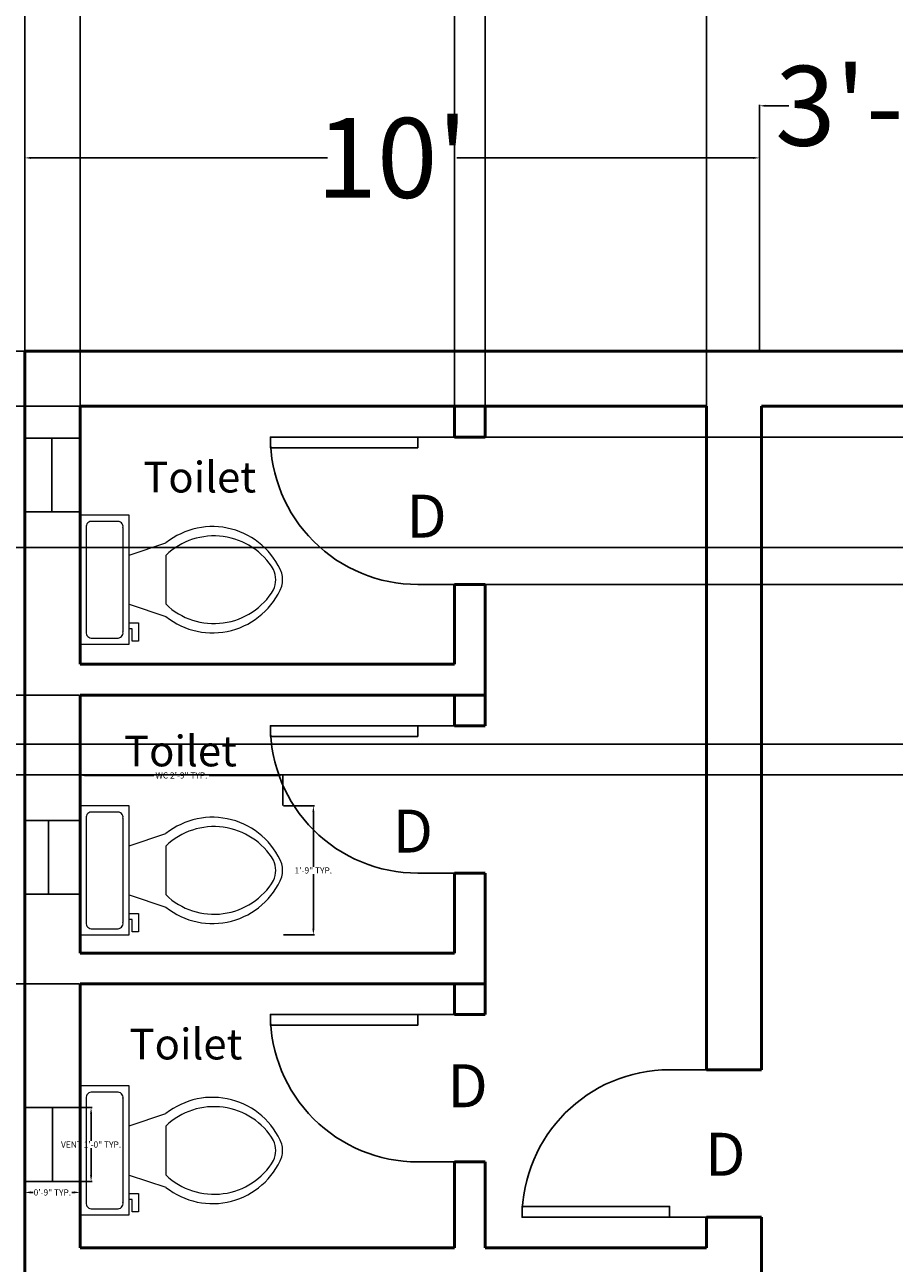
# Model space of a CAD drawing. Units: inches. Extents: x -364 to 705, y -52 to 1250.
# Tile 25 of 34: x 29 to 170, y 838 to 1039. Entities that reach past the tile are written whole.
import ezdxf

# ---------------------------------------------------------------- set-up
doc = ezdxf.new("R2010")
doc.units = ezdxf.units.IN
doc.header["$MEASUREMENT"] = 0
for name, color, linetype, lineweight in [('A-ANNO-DIMS', 4, 'Continuous', 18), ('A-ANNO-IDEN', 1, 'Continuous', 18), ('A-AREA-IDEN', 3, 'Continuous', 18), ('A-DOOR', 1, 'Continuous', 25), ('A-FLOR-FIXT', 9, 'Continuous', 18), ('A-GLAZ', 4, 'Continuous', 25), ('A-WALL', 41, 'Continuous', 50)]:
    doc.layers.add(name, color=color, linetype=linetype, lineweight=lineweight)
doc.styles.get("Standard").update_dxf_attribs({"font": 'arial.ttf'})
doc.dimstyles.get("Standard").update_dxf_attribs({"dimtxt": 1, "dimasz": 1, "dimexe": 0.18, "dimexo": 0.0625, "dimgap": 0.09, "dimtad": 0, "dimtih": 1, "dimtoh": 1, "dimdec": 0, "dimzin": 0, "dimdsep": 46, "dimlunit": 3, "dimtxsty": 'Standard', "dimcen": 0.09, "dimadec": 0, "dimazin": 0, "dimtfac": 1, "dimtdec": 0, "dimtofl": 0, "dimtmove": 0, "dimatfit": 3, "dimfxl": 1, "dimtolj": 1, "dimtzin": 0, "dimarcsym": 0})

# ---------------------------------------------------------------- blocks, each defined once
blk = doc.blocks.new('*U15')
for p, q in [((0, 0), (0, 6)), ((24, 0), (24, 6))]:
    blk.add_line(p, q)
blk.add_lwpolyline([(0, 0), (0, -24), (1.75, -24), (1.75, 0)], close=True)
blk.add_arc((0, 0), 24, 270, 0)
blk = doc.blocks.new('*U16')
for p, q in [((-24, 0), (-24, 6)), ((0, 0), (0, 6))]:
    blk.add_line(p, q)
blk.add_lwpolyline([(0, 0), (0, -24), (-1.75, -24), (-1.75, 0)], close=True)
blk.add_arc((0, 0), 24, 180, 270)
blk = doc.blocks.new('Toilet - top')
for p, q in [((9.5, -6), (9.5, -2)), ((-8, -8.5), (-8, -8)), ((-7, -8), (-7, -9.5)), ((-4, -8), (-6, -14)), ((4, -8), (6, -14)), ((-10, -8.5), (-8, -8.5)), ((-10, -9.5), (-10, -8.5)), ((-7, -9.5), (-10, -9.5)), ((4, -14), (-4, -14))]:
    blk.add_line(p, q)
blk.add_lwpolyline([(10.5, -8), (10.5, 0), (-10.5, 0), (-10.5, -8)], close=True)
for points in [[(-9.5, -2), (-9.5, -6)], [(8.5, -1), (-8.5, -1)], [(-8.5, -7), (8.5, -7)]]:
    blk.add_lwpolyline(points)
for centre, radius, start, end in [((-8.62, -1.88), 0.884, 81.8699, 188.1301), ((8.62, -1.88), 0.884, 351.8699, 98.1301), ((-8.62, -6.12), 0.884, 171.8699, 278.1301), ((8.62, -6.12), 0.884, 261.8699, 8.1301), ((3.52, -21.58), 12.17, 141.4691, 247.9714), ((4.2, -21.82), 11.33, 136.3677, 238.9468), ((-3.52, -21.58), 12.17, 292.0284, 38.5307), ((-4.2, -21.82), 11.33, 301.053, 43.6321), ((0, -27.88), 4, 245.7318, 294.2682), ((0, -29), 4, 254.8605, 285.1395)]:
    blk.add_arc(centre, radius, start, end)
blk = doc.blocks.new('*D19')
at = {"layer": 'A-ANNO-DIMS', "color": 0, "lineweight": -2, "transparency": 16777216}
for p, q in [((28.52, 986.11), (-248.33, 986.11)), ((-248.15, 985.11), (-248.15, 574.22)), ((-248.15, 149.87), (-248.15, 560.77)), ((28.52, 148.87), (-248.33, 148.87))]:
    blk.add_line(p, q, dxfattribs=at)
at = {"layer": 'A-ANNO-DIMS', "color": 0, "transparency": 16777216}
for points in [[(-248.32, 985.11), (-247.99, 985.11), (-248.15, 986.11)], [(-248.32, 149.87), (-247.99, 149.87), (-248.15, 148.87)]]:
    blk.add_solid(points, dxfattribs=at)
at = {"layer": 'Defpoints', "color": 0, "transparency": 16777216}
for p in [(28.58, 986.11), (-248.15, 148.87), (28.58, 148.87)]:
    blk.add_point(p, dxfattribs=at)
at = {"layer": 'A-ANNO-DIMS', "color": 0, "transparency": 16777216, "insert": (-248.15, 567.49), "char_height": 1, "attachment_point": 5}
blk.add_mtext('\\A1;{\\H13x;69\'-9"}', dxfattribs=at)
blk = doc.blocks.new('*D20')
at = {"layer": 'A-ANNO-DIMS', "color": 0, "lineweight": -2, "transparency": 16777216}
for p, q in [((28.52, 986.11), (-188.21, 986.11)), ((-188.03, 985.11), (-188.03, 917.23)), ((-188.03, 836.11), (-188.03, 904)), ((37.52, 835.11), (-188.21, 835.11))]:
    blk.add_line(p, q, dxfattribs=at)
at = {"layer": 'A-ANNO-DIMS', "color": 0, "transparency": 16777216}
for points in [[(-188.19, 985.11), (-187.86, 985.11), (-188.03, 986.11)], [(-188.19, 836.11), (-187.86, 836.11), (-188.03, 835.11)]]:
    blk.add_solid(points, dxfattribs=at)
at = {"layer": 'Defpoints', "color": 0, "transparency": 16777216}
for p in [(28.58, 986.11), (-188.03, 835.11), (37.58, 835.11)]:
    blk.add_point(p, dxfattribs=at)
at = {"layer": 'A-ANNO-DIMS', "color": 0, "transparency": 16777216, "insert": (-188.03, 910.61), "char_height": 1, "attachment_point": 5}
blk.add_mtext('\\A1;{\\H13x;12\'-7"}', dxfattribs=at)
blk = doc.blocks.new('*D23')
at = {"layer": 'A-ANNO-DIMS', "color": 0, "lineweight": -2, "transparency": 16777216}
for p, q in [((28.58, 986.18), (28.58, 1127.53)), ((29.58, 1127.35), (265.4, 1127.35)), ((546.58, 1127.35), (310.76, 1127.35)), ((547.58, 986.18), (547.58, 1127.53))]:
    blk.add_line(p, q, dxfattribs=at)
at = {"layer": 'A-ANNO-DIMS', "color": 0, "transparency": 16777216}
for points in [[(29.58, 1127.52), (29.58, 1127.18), (28.58, 1127.35)], [(546.58, 1127.52), (546.58, 1127.18), (547.58, 1127.35)]]:
    blk.add_solid(points, dxfattribs=at)
at = {"layer": 'Defpoints', "color": 0, "transparency": 16777216}
for p in [(547.58, 1127.35), (28.58, 986.11), (547.58, 986.11)]:
    blk.add_point(p, dxfattribs=at)
at = {"layer": 'A-ANNO-DIMS', "color": 0, "transparency": 16777216, "insert": (288.08, 1127.35), "char_height": 1, "attachment_point": 5}
blk.add_mtext('\\A1;{\\H13x;43\'-3"}', dxfattribs=at)
blk = doc.blocks.new('*D24')
at = {"layer": 'A-ANNO-DIMS', "color": 0, "lineweight": -2, "transparency": 16777216}
for p, q in [((28.58, 986.18), (28.58, 1017.73)), ((29.58, 1017.55), (77.9, 1017.55)), ((147.24, 1017.55), (98.92, 1017.55)), ((148.24, 986.18), (148.24, 1017.73))]:
    blk.add_line(p, q, dxfattribs=at)
at = {"layer": 'A-ANNO-DIMS', "color": 0, "transparency": 16777216}
for points in [[(29.58, 1017.72), (29.58, 1017.38), (28.58, 1017.55)], [(147.24, 1017.72), (147.24, 1017.38), (148.24, 1017.55)]]:
    blk.add_solid(points, dxfattribs=at)
at = {"layer": 'Defpoints', "color": 0, "transparency": 16777216}
for p in [(148.24, 1017.55), (28.58, 986.11), (148.24, 986.11)]:
    blk.add_point(p, dxfattribs=at)
at = {"layer": 'A-ANNO-DIMS', "color": 0, "transparency": 16777216, "insert": (88.41, 1017.55), "char_height": 1, "attachment_point": 5}
blk.add_mtext("\\A1;{\\H13x;10'}", dxfattribs=at)
blk = doc.blocks.new('*D25')
at = {"layer": 'A-ANNO-DIMS', "color": 0, "lineweight": -2, "transparency": 16777216}
for p, q in [((148.24, 986.18), (148.24, 1026.21)), ((192.5, 986.18), (192.5, 1026.21)), ((149.24, 1026.03), (153.01, 1026.03)), ((191.5, 1026.03), (187.73, 1026.03))]:
    blk.add_line(p, q, dxfattribs=at)
at = {"layer": 'A-ANNO-DIMS', "color": 0, "transparency": 16777216}
for points in [[(149.24, 1026.2), (149.24, 1025.86), (148.24, 1026.03)], [(191.5, 1026.2), (191.5, 1025.86), (192.5, 1026.03)]]:
    blk.add_solid(points, dxfattribs=at)
at = {"layer": 'Defpoints', "color": 0, "transparency": 16777216}
for p in [(192.5, 1026.03), (148.24, 986.11), (192.5, 986.11)]:
    blk.add_point(p, dxfattribs=at)
at = {"layer": 'A-ANNO-DIMS', "color": 0, "transparency": 16777216, "insert": (170.37, 1026.03), "char_height": 1, "attachment_point": 5}
blk.add_mtext('\\A1;{\\H13x;3\'-8"}', dxfattribs=at)
blk = doc.blocks.new('VENT-12')
blk.add_line((4.51, 0), (4.51, 12))
blk.add_lwpolyline([(9, 0), (9, 12), (0, 12), (0, 0)], close=True)
blk = doc.blocks.new('*D68')
at = {"layer": 'A-ANNO-DIMS', "color": 0, "lineweight": -2, "transparency": 16777216}
for p, q in [((37.58, 912.12), (37.58, 917.2)), ((38.58, 917.02), (49.59, 917.02)), ((69.63, 917.02), (58.62, 917.02)), ((70.63, 912.12), (70.63, 917.2))]:
    blk.add_line(p, q, dxfattribs=at)
at = {"layer": 'A-ANNO-DIMS', "color": 0, "transparency": 16777216}
for points in [[(38.58, 917.18), (38.58, 916.85), (37.58, 917.02)], [(69.63, 917.18), (69.63, 916.85), (70.63, 917.02)]]:
    blk.add_solid(points, dxfattribs=at)
at = {"layer": 'Defpoints', "color": 0, "transparency": 16777216}
for p in [(37.58, 917.02), (37.58, 912.06), (70.63, 912.06)]:
    blk.add_point(p, dxfattribs=at)
at = {"layer": 'A-ANNO-DIMS', "color": 0, "transparency": 16777216, "insert": (54.1, 917.02), "char_height": 1, "attachment_point": 5}
blk.add_mtext('\\A1;WC 2\'-9" TYP.', dxfattribs=at)
blk = doc.blocks.new('*D69')
at = {"layer": 'A-ANNO-DIMS', "color": 0, "lineweight": -2, "transparency": 16777216}
for p, q in [((70.69, 912.06), (75.76, 912.06)), ((75.58, 911.06), (75.58, 902.16)), ((75.58, 892.06), (75.58, 900.96)), ((70.69, 891.06), (75.76, 891.06))]:
    blk.add_line(p, q, dxfattribs=at)
at = {"layer": 'A-ANNO-DIMS', "color": 0, "transparency": 16777216}
for points in [[(75.42, 911.06), (75.75, 911.06), (75.58, 912.06)], [(75.42, 892.06), (75.75, 892.06), (75.58, 891.06)]]:
    blk.add_solid(points, dxfattribs=at)
at = {"layer": 'Defpoints', "color": 0, "transparency": 16777216}
for p in [(70.63, 912.06), (75.58, 912.06), (70.63, 891.06)]:
    blk.add_point(p, dxfattribs=at)
at = {"layer": 'A-ANNO-DIMS', "color": 0, "transparency": 16777216, "insert": (75.58, 901.56), "char_height": 1, "attachment_point": 5}
blk.add_mtext('\\A1;1\'-9" TYP.', dxfattribs=at)
blk = doc.blocks.new('*D74')
at = {"layer": 'A-ANNO-DIMS', "color": 0, "lineweight": -2, "transparency": 16777216}
for p, q in [((37.64, 862.94), (39.56, 862.94)), ((39.38, 861.94), (39.38, 857.54)), ((39.38, 851.94), (39.38, 856.34)), ((37.64, 850.94), (39.56, 850.94))]:
    blk.add_line(p, q, dxfattribs=at)
at = {"layer": 'A-ANNO-DIMS', "color": 0, "transparency": 16777216}
for points in [[(39.21, 861.94), (39.55, 861.94), (39.38, 862.94)], [(39.21, 851.94), (39.55, 851.94), (39.38, 850.94)]]:
    blk.add_solid(points, dxfattribs=at)
at = {"layer": 'Defpoints', "color": 0, "transparency": 16777216}
for p in [(37.58, 862.94), (39.38, 862.94), (37.58, 850.94)]:
    blk.add_point(p, dxfattribs=at)
at = {"layer": 'A-ANNO-DIMS', "color": 0, "transparency": 16777216, "insert": (39.38, 856.94), "char_height": 1, "attachment_point": 5}
blk.add_mtext('\\A1;VENT 1\'-0" TYP.', dxfattribs=at)
blk = doc.blocks.new('*D75')
at = {"layer": 'A-ANNO-DIMS', "color": 0, "lineweight": -2, "transparency": 16777216}
for p, q in [((28.58, 850.88), (28.58, 848.96)), ((37.58, 850.88), (37.58, 848.96)), ((29.58, 849.14), (29.94, 849.14)), ((36.58, 849.14), (36.22, 849.14))]:
    blk.add_line(p, q, dxfattribs=at)
at = {"layer": 'A-ANNO-DIMS', "color": 0, "transparency": 16777216}
for points in [[(29.58, 849.31), (29.58, 848.98), (28.58, 849.14)], [(36.58, 849.31), (36.58, 848.98), (37.58, 849.14)]]:
    blk.add_solid(points, dxfattribs=at)
at = {"layer": 'Defpoints', "color": 0, "transparency": 16777216}
for p in [(28.58, 850.94), (37.58, 850.94), (37.58, 849.14)]:
    blk.add_point(p, dxfattribs=at)
at = {"layer": 'A-ANNO-DIMS', "color": 0, "transparency": 16777216, "insert": (33.08, 849.14), "char_height": 1, "attachment_point": 5}
blk.add_mtext('\\A1;0\'-9" TYP.', dxfattribs=at)
blk = doc.blocks.new('*D91')
at = {"layer": 'A-ANNO-DIMS', "color": 0, "lineweight": -2, "transparency": 16777216}
for p, q in [((37.58, 977.18), (37.58, 1141.54)), ((38.58, 1141.36), (66.66, 1141.36)), ((97.58, 1141.36), (69.5, 1141.36)), ((98.58, 977.18), (98.58, 1141.54))]:
    blk.add_line(p, q, dxfattribs=at)
at = {"layer": 'A-ANNO-DIMS', "color": 0, "transparency": 16777216}
for points in [[(38.58, 1141.53), (38.58, 1141.2), (37.58, 1141.36)], [(97.58, 1141.53), (97.58, 1141.2), (98.58, 1141.36)]]:
    blk.add_solid(points, dxfattribs=at)
at = {"layer": 'Defpoints', "color": 0, "transparency": 16777216}
for p in [(98.58, 1141.36), (37.58, 977.11), (98.58, 977.11)]:
    blk.add_point(p, dxfattribs=at)
at = {"layer": 'A-ANNO-DIMS', "color": 0, "transparency": 16777216, "insert": (68.08, 1141.36), "char_height": 1, "attachment_point": 5}
blk.add_mtext('\\A1;5\'-1"', dxfattribs=at)
blk = doc.blocks.new('*D92')
at = {"layer": 'A-ANNO-DIMS', "color": 0, "lineweight": -2, "transparency": 16777216}
for p, q in [((103.58, 977.18), (103.58, 1141.54)), ((104.58, 1141.36), (120.16, 1141.36)), ((138.58, 1141.36), (123, 1141.36)), ((139.58, 977.18), (139.58, 1141.54))]:
    blk.add_line(p, q, dxfattribs=at)
at = {"layer": 'A-ANNO-DIMS', "color": 0, "transparency": 16777216}
for points in [[(104.58, 1141.53), (104.58, 1141.2), (103.58, 1141.36)], [(138.58, 1141.53), (138.58, 1141.2), (139.58, 1141.36)]]:
    blk.add_solid(points, dxfattribs=at)
at = {"layer": 'Defpoints', "color": 0, "transparency": 16777216}
for p in [(139.58, 1141.36), (103.58, 977.11), (139.58, 977.11)]:
    blk.add_point(p, dxfattribs=at)
at = {"layer": 'A-ANNO-DIMS', "color": 0, "transparency": 16777216, "insert": (121.58, 1141.36), "char_height": 1, "attachment_point": 5}
blk.add_mtext('\\A1;3\'-0"', dxfattribs=at)
blk = doc.blocks.new('*D93')
at = {"layer": 'A-ANNO-DIMS', "color": 0, "lineweight": -2, "transparency": 16777216}
for p, q in [((37.52, 977.11), (-126.85, 977.11)), ((-126.67, 976.11), (-126.67, 954.22)), ((-126.67, 931.11), (-126.67, 953.01)), ((37.52, 930.11), (-126.85, 930.11))]:
    blk.add_line(p, q, dxfattribs=at)
at = {"layer": 'A-ANNO-DIMS', "color": 0, "transparency": 16777216}
for points in [[(-126.84, 976.11), (-126.5, 976.11), (-126.67, 977.11)], [(-126.84, 931.11), (-126.5, 931.11), (-126.67, 930.11)]]:
    blk.add_solid(points, dxfattribs=at)
at = {"layer": 'Defpoints', "color": 0, "transparency": 16777216}
for p in [(37.58, 977.11), (-126.67, 930.11), (37.58, 930.11)]:
    blk.add_point(p, dxfattribs=at)
at = {"layer": 'A-ANNO-DIMS', "color": 0, "transparency": 16777216, "insert": (-126.67, 953.61), "char_height": 1, "attachment_point": 5}
blk.add_mtext('\\A1;3\'-11"', dxfattribs=at)
blk = doc.blocks.new('*D94')
at = {"layer": 'A-ANNO-DIMS', "color": 0, "lineweight": -2, "transparency": 16777216}
for p, q in [((37.52, 930.11), (-126.85, 930.11)), ((-126.67, 929.11), (-126.67, 907.22)), ((-126.67, 884.11), (-126.67, 906.01)), ((37.52, 883.11), (-126.85, 883.11))]:
    blk.add_line(p, q, dxfattribs=at)
at = {"layer": 'A-ANNO-DIMS', "color": 0, "transparency": 16777216}
for points in [[(-126.84, 929.11), (-126.5, 929.11), (-126.67, 930.11)], [(-126.84, 884.11), (-126.5, 884.11), (-126.67, 883.11)]]:
    blk.add_solid(points, dxfattribs=at)
at = {"layer": 'Defpoints', "color": 0, "transparency": 16777216}
for p in [(37.58, 930.11), (-126.67, 883.11), (37.58, 883.11)]:
    blk.add_point(p, dxfattribs=at)
at = {"layer": 'A-ANNO-DIMS', "color": 0, "transparency": 16777216, "insert": (-126.67, 906.61), "char_height": 1, "attachment_point": 5}
blk.add_mtext('\\A1;3\'-11"', dxfattribs=at)
blk = doc.blocks.new('*D95')
at = {"layer": 'A-ANNO-DIMS', "color": 0, "lineweight": -2, "transparency": 16777216}
for p, q in [((103.64, 972.11), (703.01, 972.11)), ((702.83, 971.11), (702.83, 960.72)), ((702.83, 949.11), (702.83, 959.51)), ((103.64, 948.11), (703.01, 948.11))]:
    blk.add_line(p, q, dxfattribs=at)
at = {"layer": 'A-ANNO-DIMS', "color": 0, "transparency": 16777216}
for points in [[(702.66, 971.11), (703, 971.11), (702.83, 972.11)], [(702.66, 949.11), (703, 949.11), (702.83, 948.11)]]:
    blk.add_solid(points, dxfattribs=at)
at = {"layer": 'Defpoints', "color": 0, "transparency": 16777216}
for p in [(103.58, 972.11), (702.83, 972.11), (103.58, 948.11)]:
    blk.add_point(p, dxfattribs=at)
at = {"layer": 'A-ANNO-DIMS', "color": 0, "transparency": 16777216, "insert": (702.83, 960.11), "char_height": 1, "attachment_point": 5}
blk.add_mtext('\\A1;2\'-0"', dxfattribs=at)
blk = doc.blocks.new('*D103')
at = {"layer": 'A-ANNO-DIMS', "color": 0, "lineweight": -2, "transparency": 16777216}
for p, q in [((193.52, 954.1), (-126.85, 954.1)), ((-126.67, 953.1), (-126.67, 938.71)), ((-126.67, 923.11), (-126.67, 937.51)), ((193.52, 922.11), (-126.85, 922.11))]:
    blk.add_line(p, q, dxfattribs=at)
at = {"layer": 'A-ANNO-DIMS', "color": 0, "transparency": 16777216}
for points in [[(-126.84, 953.1), (-126.5, 953.1), (-126.67, 954.1)], [(-126.84, 923.11), (-126.5, 923.11), (-126.67, 922.11)]]:
    blk.add_solid(points, dxfattribs=at)
at = {"layer": 'Defpoints', "color": 0, "transparency": 16777216}
for p in [(-126.67, 954.1), (193.58, 954.1), (193.58, 922.11)]:
    blk.add_point(p, dxfattribs=at)
at = {"layer": 'A-ANNO-DIMS', "color": 0, "transparency": 16777216, "insert": (-126.67, 938.11), "char_height": 1, "attachment_point": 5}
blk.add_mtext('\\A1;2\'-8"', dxfattribs=at)
blk = doc.blocks.new('*D104')
at = {"layer": 'A-ANNO-DIMS', "color": 0, "lineweight": -2, "transparency": 16777216}
for p, q in [((193.52, 922.11), (-126.85, 922.11)), ((-126.67, 921.11), (-126.67, 920.22)), ((-126.67, 918.11), (-126.67, 919.01)), ((193.52, 917.11), (-126.85, 917.11))]:
    blk.add_line(p, q, dxfattribs=at)
at = {"layer": 'A-ANNO-DIMS', "color": 0, "transparency": 16777216}
for points in [[(-126.84, 921.11), (-126.5, 921.11), (-126.67, 922.11)], [(-126.84, 918.11), (-126.5, 918.11), (-126.67, 917.11)]]:
    blk.add_solid(points, dxfattribs=at)
at = {"layer": 'Defpoints', "color": 0, "transparency": 16777216}
for p in [(-126.67, 922.11), (193.58, 922.11), (193.58, 917.11)]:
    blk.add_point(p, dxfattribs=at)
at = {"layer": 'A-ANNO-DIMS', "color": 0, "transparency": 16777216, "insert": (-126.67, 919.61), "char_height": 1, "attachment_point": 5}
blk.add_mtext('\\A1;0\'-5"', dxfattribs=at)

msp = doc.modelspace()

# ---------------------------------------------------------------- linework, layer by layer
at = {"layer": 'A-GLAZ'}
for p, q in [((32.99, 959.92), (32.99, 971.92)), ((32.43, 897.68), (32.43, 909.68))]:
    msp.add_line(p, q, dxfattribs=at)
for points in [[(37.58, 959.92), (37.58, 971.92), (28.58, 971.92), (28.58, 959.92)], [(37.58, 897.68), (37.58, 909.68), (28.58, 909.68), (28.58, 897.68)]]:
    msp.add_lwpolyline(points, close=True, dxfattribs=at)
at = {"layer": 'A-WALL'}
for p, q in [((547.58, 986.11), (28.58, 986.11)), ((28.58, 11.11), (28.58, 986.11)), ((37.58, 935.11), (37.58, 977.11)), ((98.58, 977.11), (37.58, 977.11)), ((98.58, 977.11), (103.58, 977.11)), ((98.58, 972.11), (98.58, 977.11)), ((139.58, 977.11), (103.58, 977.11)), ((103.58, 972.11), (103.58, 977.11)), ((139.58, 869.11), (139.58, 977.11)), ((184.58, 977.11), (148.58, 977.11)), ((148.58, 869.11), (148.58, 977.11)), ((98.58, 972.11), (103.58, 972.11)), ((98.58, 935.11), (98.58, 948.11)), ((98.58, 948.11), (103.58, 948.11)), ((103.58, 925.11), (103.58, 948.11)), ((98.58, 935.11), (37.58, 935.11)), ((98.58, 930.11), (37.58, 930.11)), ((37.58, 888.11), (37.58, 930.11)), ((98.58, 930.11), (103.58, 930.11)), ((98.58, 925.11), (98.58, 930.11)), ((98.58, 925.11), (103.58, 925.11)), ((98.58, 888.11), (98.58, 901.11)), ((98.58, 901.11), (103.58, 901.11)), ((103.58, 878.11), (103.58, 901.11)), ((98.58, 888.11), (37.58, 888.11)), ((98.58, 883.11), (37.58, 883.11)), ((37.58, 840.11), (37.58, 883.11)), ((98.58, 883.11), (103.58, 883.11)), ((98.58, 878.11), (98.58, 883.11)), ((98.58, 878.11), (103.58, 878.11)), ((139.58, 869.11), (148.58, 869.11)), ((98.58, 840.11), (98.58, 854.11)), ((98.58, 854.11), (103.58, 854.11)), ((103.58, 840.11), (103.58, 854.11)), ((139.58, 840.11), (139.58, 845.11)), ((139.58, 845.11), (148.58, 845.11)), ((148.58, 830.11), (148.58, 845.11)), ((98.58, 840.11), (37.58, 840.11)), ((139.58, 840.11), (103.58, 840.11))]:
    msp.add_line(p, q, dxfattribs=at)

# ---------------------------------------------------------------- block references
at = {"layer": 'A-DOOR', "rotation": 270}
for name, p in [('*U15', (92.58, 972.11)), ('*U15', (92.58, 925.11)), ('*U15', (92.58, 878.11)), ('*U16', (133.58, 845.11))]:
    msp.add_blockref(name, p, dxfattribs=at)
at = {"layer": 'A-FLOR-FIXT'}
for p, rotation in [((37.58, 948.88), 89.99999999999999), ((37.58, 901.56), 90), ((37.58, 855.97), 90)]:
    msp.add_blockref('Toilet - top', p, dxfattribs=dict(at, rotation=rotation))
at = {"layer": 'A-GLAZ'}
msp.add_blockref('VENT-12', (28.58, 850.94), dxfattribs=at)

# ---------------------------------------------------------------- texts
at = {"layer": 'A-ANNO-IDEN', "char_height": 7, "attachment_point": 1}
for insert in [(90.72, 962.73), (88.49, 911.46), (97.41, 870), (139.37, 858.85)]:
    msp.add_mtext_dynamic_manual_height_columns('D', width=150.7943, gutter_width=1, heights=[0], dxfattribs=dict(at, insert=insert))
at = {"layer": 'A-AREA-IDEN', "char_height": 5, "attachment_point": 1}
for insert in [(47.87, 968.08), (44.74, 923.5), (45.64, 875.79)]:
    msp.add_mtext_dynamic_manual_height_columns('Toilet', width=150.7943, gutter_width=1, heights=[0], dxfattribs=dict(at, insert=insert))

# ---------------------------------------------------------------- dimensions: what is measured, and where the dimension line sits
at = {"layer": 'A-ANNO-DIMS'}
for base, p1, p2, picture, middle in [((98.58, 1141.36), (37.58, 977.11), (98.58, 977.11), '*D91', (68.08, 1141.36)), ((139.58, 1141.36), (103.58, 977.11), (139.58, 977.11), '*D92', (121.58, 1141.36))]:
    dim = msp.add_linear_dim(base=base, p1=p1, p2=p2, dimstyle='Standard', override={"dimdec": 1, "dimlfac": 1, "dimrnd": 0, "dimzin": 1, "dimdsep": 46, "dimlunit": 4, "dimfrac": 2}, dxfattribs=at)
    dim.commit()
    dim.dimension.update_dxf_attribs({"geometry": picture, "text_midpoint": middle})
for base, p1, p2, text, override, picture, middle in [((547.58, 1127.35), (28.58, 986.11), (547.58, 986.11), '{\\H13x;<>}', {"dimclrd": 0, "dimclre": 0, "dimclrt": 0}, '*D23', (288.08, 1127.35)), ((192.5, 1026.03), (148.24, 986.11), (192.5, 986.11), '{\\H13x;<>}', {"dimclrd": 0, "dimclre": 0, "dimclrt": 0}, '*D25', (170.37, 1026.03)), ((148.24, 1017.55), (28.58, 986.11), (148.24, 986.11), '{\\H13x;<>}', {"dimclrd": 0, "dimclre": 0, "dimclrt": 0}, '*D24', (88.41, 1017.55)), ((37.58, 849.14), (28.58, 850.94), (37.58, 850.94), '<> TYP.', {"dimdec": 1, "dimlfac": 1, "dimrnd": 0, "dimzin": 1, "dimdsep": 46, "dimlunit": 4, "dimfrac": 2}, '*D75', (33.08, 849.14))]:
    dim = msp.add_linear_dim(base=base, p1=p1, p2=p2, text=text, dimstyle='Standard', override=override, dxfattribs=at)
    dim.commit()
    dim.dimension.update_dxf_attribs({"geometry": picture, "text_midpoint": middle})
for base, p1, p2, angle, text, override, picture, middle in [((-248.15, 148.87), (28.58, 986.11), (28.58, 148.87), 90, '{\\H13x;<>}', {"dimclrd": 0, "dimclre": 0, "dimclrt": 0}, '*D19', (-248.15, 567.49)), ((37.5805, 917.0168), (70.6268, 912.0599), (37.5805, 912.0599), 180, 'WC <> TYP.', {"dimdec": 1, "dimlfac": 1, "dimrnd": 0, "dimzin": 1, "dimdsep": 46, "dimlunit": 4, "dimfrac": 2}, '*D68', (54.1037, 917.0168)), ((75.58, 912.06), (70.63, 891.06), (70.63, 912.06), 90, '<> TYP.', {"dimdec": 1, "dimlfac": 1, "dimrnd": 0, "dimzin": 1, "dimdsep": 46, "dimlunit": 4, "dimfrac": 2}, '*D69', (75.58, 901.56)), ((39.38, 862.94), (37.58, 850.94), (37.58, 862.94), 90, 'VENT <> TYP.', {"dimdec": 1, "dimlfac": 1, "dimrnd": 0, "dimzin": 1, "dimdsep": 46, "dimlunit": 4, "dimfrac": 2}, '*D74', (39.38, 856.94))]:
    dim = msp.add_linear_dim(base=base, p1=p1, p2=p2, angle=angle, text=text, dimstyle='Standard', override=override, dxfattribs=at)
    dim.commit()
    dim.dimension.update_dxf_attribs({"geometry": picture, "text_midpoint": middle})
dim = msp.add_linear_dim(base=(-188.03, 835.11), p1=(28.58, 986.11), p2=(37.58, 835.11), angle=90, text='{\\H13x;<>}', dimstyle='Standard', override={"dimclrd": 0, "dimclre": 0, "dimclrt": 0}, dxfattribs=at)
dim.commit()
dim.dimension.update_dxf_attribs({"geometry": '*D20', "text_midpoint": (-188.03, 910.61), "dimtype": 160})
for base, p1, p2, picture, middle in [((-126.67, 930.11), (37.58, 977.11), (37.58, 930.11), '*D93', (-126.67, 953.61)), ((702.83, 972.11), (103.58, 948.11), (103.58, 972.11), '*D95', (702.83, 960.11)), ((-126.67, 954.1), (193.58, 922.11), (193.58, 954.1), '*D103', (-126.67, 938.11)), ((-126.67, 883.11), (37.58, 930.11), (37.58, 883.11), '*D94', (-126.67, 906.61)), ((-126.67, 922.11), (193.58, 917.11), (193.58, 922.11), '*D104', (-126.67, 919.61))]:
    dim = msp.add_linear_dim(base=base, p1=p1, p2=p2, angle=90, dimstyle='Standard', override={"dimdec": 1, "dimlfac": 1, "dimrnd": 0, "dimzin": 1, "dimdsep": 46, "dimlunit": 4, "dimfrac": 2}, dxfattribs=at)
    dim.commit()
    dim.dimension.update_dxf_attribs({"geometry": picture, "text_midpoint": middle})

doc.saveas('drawing.dxf')
